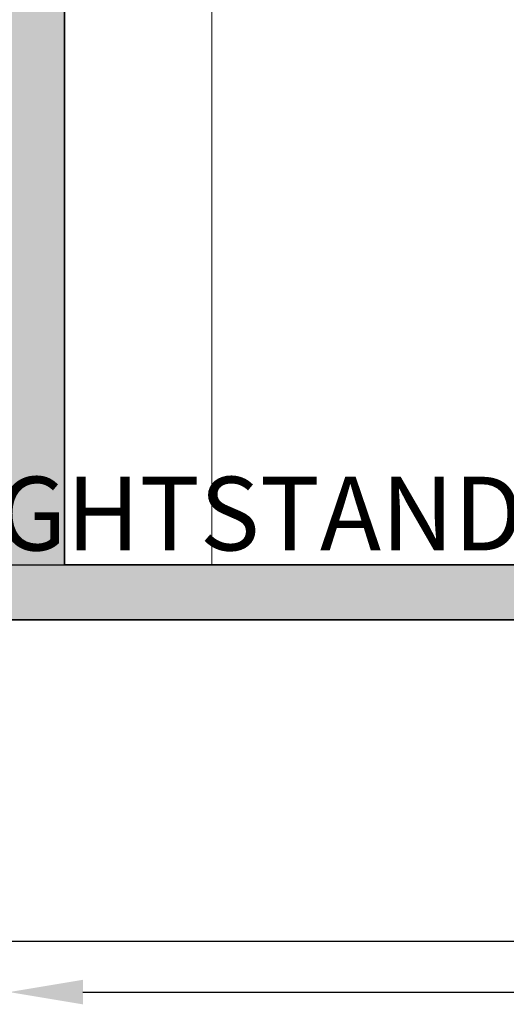
# Model space of a CAD drawing. Units: inches. Extents: x 2083 to 3317, y 1141 to 2115.
# Tile 111 of 256: x 2865 to 2944, y 1201 to 1361. Entities that reach past the tile are written whole.
import ezdxf

# ---------------------------------------------------------------- set-up
doc = ezdxf.new("R2010")
doc.units = ezdxf.units.IN
for name, color, linetype, lineweight in [('A-ANNO-DIMS', 2, 'Continuous', 18), ('A-FLOR-CASE', 8, 'Continuous', 18), ('A-WALL', 7, 'Continuous', 35)]:
    doc.layers.add(name, color=color, linetype=linetype, lineweight=lineweight)
doc.layers.add('A-WALL-PATT', color=251, linetype='Continuous', lineweight=13, true_color=0x636466)
doc.styles.get("Standard").update_dxf_attribs({"font": 'arial.ttf'})
doc.dimstyles.new('ISO-25', dxfattribs={"dimtxt": 12, "dimasz": 12, "dimexe": 1.25, "dimexo": 0.625, "dimtad": 1, "dimlunit": 3, "dimtxsty": 'Standard', "dimcen": 2.5, "dimadec": 0, "dimazin": 0, "dimtfac": 1, "dimtmove": 0, "dimatfit": 3, "dimfxl": 1, "dimarcsym": 0})

# ---------------------------------------------------------------- blocks, each defined once
blk = doc.blocks.new('*D10')
at = {"layer": 'A-ANNO-DIMS', "color": 0, "lineweight": -2, "transparency": 16777216}
for p, q in [((2862.96, 1262.64), (2862.96, 1201.38)), ((3126.96, 1262.64), (3126.96, 1201.38)), ((2874.96, 1202.63), (3114.96, 1202.63))]:
    blk.add_line(p, q, dxfattribs=at)
at = {"layer": 'A-ANNO-DIMS', "color": 0, "transparency": 16777216}
for points in [[(2874.96, 1204.63), (2874.96, 1200.63), (2862.96, 1202.63)], [(3114.96, 1204.63), (3114.96, 1200.63), (3126.96, 1202.63)]]:
    blk.add_solid(points, dxfattribs=at)
at = {"layer": 'Defpoints', "color": 0, "transparency": 16777216}
for p in [(2862.96, 1263.26), (3126.96, 1263.26), (3126.96, 1202.63)]:
    blk.add_point(p, dxfattribs=at)
at = {"layer": 'A-ANNO-DIMS', "color": 0, "transparency": 16777216, "insert": (2994.96, 1209.28), "char_height": 12, "attachment_point": 5}
blk.add_mtext("22'", dxfattribs=at)
blk = doc.blocks.new('CASEWORK-96X24')
for q in [(0, 0), (24, 96)]:
    blk.add_line((0, 96), q)
blk = doc.blocks.new('*D26')
at = {"layer": 'A-ANNO-DIMS', "color": 0, "lineweight": -2, "transparency": 16777216}
for p, q in [((3088.99, 1274.92), (3088.99, 1270.95)), ((3111.24, 1274.92), (3111.24, 1270.95)), ((3076.99, 1272.2), (2840.26, 1272.2)), ((3111.24, 1272.2), (3088.99, 1272.2)), ((3123.24, 1272.2), (3135.24, 1272.2))]:
    blk.add_line(p, q, dxfattribs=at)
at = {"layer": 'A-ANNO-DIMS', "color": 0, "transparency": 16777216}
for points in [[(3076.99, 1274.2), (3076.99, 1270.2), (3088.99, 1272.2)], [(3123.24, 1274.2), (3123.24, 1270.2), (3111.24, 1272.2)]]:
    blk.add_solid(points, dxfattribs=at)
at = {"layer": 'Defpoints', "color": 0, "transparency": 16777216}
for p in [(3088.99, 1275.54), (3111.24, 1275.54), (3088.99, 1272.2)]:
    blk.add_point(p, dxfattribs=at)
at = {"layer": 'A-ANNO-DIMS', "color": 0, "transparency": 16777216, "insert": (2952.62, 1279.03), "char_height": 12, "attachment_point": 5}
blk.add_mtext('NIGHTSTAND 1\'-10 1/2" TYP.', dxfattribs=at)
blk = doc.blocks.new('*D34')
at = {"layer": 'A-ANNO-DIMS', "color": 0, "lineweight": -2, "transparency": 16777216}
for p, q in [((2226.96, 1262.64), (2226.96, 1209.66)), ((3126.96, 1262.64), (3126.96, 1209.66)), ((2238.96, 1210.91), (3114.96, 1210.91))]:
    blk.add_line(p, q, dxfattribs=at)
at = {"layer": 'A-ANNO-DIMS', "color": 0, "transparency": 16777216}
for points in [[(2238.96, 1212.91), (2238.96, 1208.91), (2226.96, 1210.91)], [(3114.96, 1212.91), (3114.96, 1208.91), (3126.96, 1210.91)]]:
    blk.add_solid(points, dxfattribs=at)
at = {"layer": 'Defpoints', "color": 0, "transparency": 16777216}
for p in [(2226.96, 1263.26), (3126.96, 1263.26), (3126.96, 1210.91)]:
    blk.add_point(p, dxfattribs=at)
at = {"layer": 'A-ANNO-DIMS', "color": 0, "transparency": 16777216, "insert": (2676.96, 1217.66), "char_height": 12, "attachment_point": 5}
blk.add_mtext('75\'-0"', dxfattribs=at)
blk = doc.blocks.new('*D73')
at = {"layer": 'A-ANNO-DIMS', "color": 0, "lineweight": -2, "transparency": 16777216}
for p, q in [((2895.87, 1420.76), (2930.55, 1387.52)), ((2980.11, 1340.03), (2939.22, 1379.22))]:
    blk.add_line(p, q, dxfattribs=at)
at = {"layer": 'A-ANNO-DIMS', "color": 0, "transparency": 16777216}
blk.add_solid([(2940.6, 1380.66), (2937.83, 1377.77), (2930.55, 1387.52)], dxfattribs=at)
at = {"layer": 'Defpoints', "color": 0, "transparency": 16777216}
for p in [(2895.87, 1420.76), (2930.55, 1387.52)]:
    blk.add_point(p, dxfattribs=at)
at = {"layer": 'A-ANNO-DIMS', "color": 0, "transparency": 16777216, "insert": (2968.66, 1360.35), "char_height": 12, "attachment_point": 5, "rotation": 316.2187}
blk.add_mtext('R4\'-0"', dxfattribs=at)

msp = doc.modelspace()

# ---------------------------------------------------------------- hatches: boundary and pattern name
at = {"layer": 'A-WALL-PATT'}
h = msp.add_hatch(color=256, dxfattribs=at)
h.dxf.hatch_style = 1
h.paths.add_polyline_path([(3126.96, 2020.761), (2748.96, 2020.761), (2604.96, 2020.761), (2226.96, 2020.761), (2226.96, 1702.761), (2466.96, 1702.761), (2466.96, 1582.761), (2418.96, 1582.761), (2418.96, 1477.761), (2226.96, 1477.761), (2226.96, 1263.261), (2544.96, 1263.261), (2544.96, 1411.761), (2604.96, 1411.761), (2685.96, 1411.761), (2685.96, 1420.761), (2604.96, 1420.761), (2604.96, 1573.761), (2604.96, 1702.761), (2604.96, 2011.761), (2748.96, 2011.761), (2748.96, 1702.761), (2862.96, 1702.761), (2862.96, 1621.761), (2871.96, 1621.761), (2871.96, 1702.761), (2883.96, 1702.761), (2883.96, 1706.939, -0.0264593), (2883.96, 1711.761), (2757.96, 1711.761), (2757.96, 1807.761), (2787.96, 1807.761), (2787.96, 1812.261), (2757.96, 1812.261), (2757.96, 2011.761), (2877.96, 2011.761), (2877.96, 1812.261), (2847.96, 1812.261), (2847.96, 1807.761), (2889.836, 1807.761), (2889.836, 1812.261), (2882.46, 1812.261), (2882.46, 2011.761), (3117.96, 2011.761), (3117.96, 1812.261), (2937.836, 1812.261), (2937.836, 1807.761), (2995.71, 1807.761), (2995.71, 1796.118), (3000.21, 1796.118), (3000.21, 1807.761), (3117.96, 1807.761), (3117.96, 1711.761), (3000.21, 1711.761), (3000.21, 1760.118), (2998.573, 1760.118, -0.020711), (2995.71, 1760.118), (2995.71, 1711.761), (2931.96, 1711.761), (2931.96, 1702.761), (3126.96, 1702.761)])
h.paths.add_polyline_path([(2471.46, 2011.761), (2471.46, 1810.011), (2462.717, 1810.011), (2462.717, 1805.511), (2505.96, 1805.511), (2505.96, 1810.011), (2475.96, 1810.011), (2475.96, 2011.761), (2595.96, 2011.761), (2595.96, 1810.011), (2565.96, 1810.011), (2565.96, 1805.511), (2595.96, 1805.511), (2595.96, 1711.761), (2235.96, 1711.761), (2235.96, 1805.511), (2353.71, 1805.511), (2353.71, 1796.054), (2358.21, 1796.054), (2358.21, 1805.511), (2414.717, 1805.511), (2414.717, 1810.011), (2235.96, 1810.011), (2235.96, 2011.761)], flags=16)
h.paths.add_polyline_path([(2270.205, 1994.61), (2270.205, 1970.61), (2246.205, 1970.61), (2246.205, 1994.61)], flags=0)
edge = h.paths.add_edge_path(flags=0)
edge.add_ellipse((2332.027, 1899.798), major_axis=(-3.043, 3.043), ratio=0.1682525, start_angle=-161.33217, end_angle=-156.30711, ccw=False)
edge.add_ellipse((2333.082, 1898.744), major_axis=(-1.055, 1.055), ratio=0.4535321, start_angle=-123.37102, end_angle=-94.15911)
edge = h.paths.add_edge_path(flags=0)
edge.add_ellipse((2332.027, 1968.876), major_axis=(3.043, 3.043), ratio=0.1682525, start_angle=18.66783, end_angle=23.69289)
edge.add_spline(control_points=[(2332.926, 1970.691), (2332.227, 1970.336), (2330.894, 1969.659), (2328.413, 1970.932), (2327.204, 1967.749), (2324.71, 1969.956), (2322.533, 1967.012), (2320.013, 1971.296), (2317.68, 1968.158), (2316.041, 1967.102), (2315.427, 1966.81)], knot_values=[0, 0, 0, 0, 2.2670587, 4.3245589, 6.6855835, 8.8786411, 11.121502, 14.300359, 17.7552837, 19.732645, 19.732645, 19.732645, 19.732645], degree=3, periodic=0)
edge.add_ellipse((2332.027, 1968.876), major_axis=(3.043, 3.043), ratio=0.1682525, start_angle=18.66783, end_angle=23.69289, ccw=False)
edge.add_ellipse((2333.082, 1969.931), major_axis=(1.055, 1.055), ratio=0.4535321, start_angle=56.62898, end_angle=85.84089, ccw=False)
edge = h.paths.add_edge_path(flags=0)
edge.add_spline(control_points=[(2296.428, 1967.988), (2293.628, 1965.336), (2287.704, 1959.727), (2299.744, 1949.996), (2294.533, 1935.669), (2290.573, 1920.604), (2293.394, 1909.974), (2296.185, 1904.967)], knot_values=[0.0991853, 0.0991853, 0.0991853, 0.0991853, 0.3453009, 0.6198217, 0.9826526, 1.3860932, 1.8105546, 1.8105546, 1.8105546, 1.8105546], degree=3, periodic=0)
edge.add_spline(control_points=[(2296.185, 1904.967), (2297.384, 1902.619), (2298.001, 1901.949), (2298.553, 1901.468)], knot_values=[0.0062457, 0.0062457, 0.0062457, 0.0062457, 0.0554759, 0.0554759, 0.0554759, 0.0554759], degree=3, periodic=0)
edge.add_spline(control_points=[(2298.553, 1901.468), (2297.259, 1900.923), (2295.225, 1900.232), (2293.06, 1900.614), (2292.101, 1900.788), (2292.09, 1900.791)], knot_values=[0.3128349, 0.3128349, 0.3128349, 0.3128349, 0.4017797, 0.4749867, 0.4759027, 0.4759027, 0.4759027, 0.4759027], degree=3, periodic=0)
edge.add_arc((2292.794, 1904.664), 3.937, 215.4209, 259.69818, ccw=False)
edge.add_spline(control_points=[(2289.585, 1902.382), (2289.477, 1902.535), (2289.368, 1902.688), (2289.261, 1902.841)], knot_values=[0.1028719, 0.1028719, 0.1028719, 0.1028719, 0.1168958, 0.1168958, 0.1168958, 0.1168958], degree=3, periodic=0)
edge.add_spline(control_points=[(2289.261, 1902.841), (2288.687, 1902.55), (2287.64, 1902.02), (2285.881, 1901.874), (2283.853, 1901.504), (2281.72, 1899.711), (2278.467, 1899.493), (2276.157, 1901.883), (2272.259, 1899.804), (2267.778, 1901.843), (2262.244, 1900.184), (2257.415, 1901.782), (2254.318, 1900.726), (2253.178, 1900.337)], knot_values=[0, 0, 0, 0, 1.9079767, 3.4771759, 5.261074, 7.9728515, 11.6802485, 13.7179214, 16.9395917, 22.789562, 27.5025027, 33.5952153, 37.1456181, 37.1456181, 37.1456181, 37.1456181], degree=3, periodic=0)
edge.add_line((2253.178, 1900.337), (2250.244, 1902.841))
edge.add_line((2250.244, 1902.841), (2250.244, 1965.833))
edge.add_line((2250.244, 1965.833), (2253.178, 1968.337))
edge.add_spline(control_points=[(2253.178, 1968.337), (2254.318, 1967.948), (2257.415, 1966.892), (2262.244, 1968.49), (2267.778, 1966.831), (2271.527, 1968.537), (2273.876, 1967.828), (2274.207, 1967.728)], knot_values=[0, 0, 0, 0, 0.0901802, 0.2449351, 0.3646438, 0.5132331, 0.5378548, 0.5378548, 0.5378548, 0.5378548], degree=3, periodic=0)
edge.add_arc((2274.353, 1963.793), 3.937, 72.05113, 92.12795, ccw=False)
edge.add_arc((2281.297, 1985.23), 18.596, 252.05113, 288.56572)
edge.add_arc((2292.317, 1956.029), 12.646, 71.02679, 113.77822, ccw=False)
edge = h.paths.add_edge_path(flags=0)
edge.add_spline(control_points=[(2274.899, 1951.856), (2275.066, 1951.617), (2275.233, 1951.377), (2275.398, 1951.136)], knot_values=[1.4099157, 1.4099157, 1.4099157, 1.4099157, 1.4315903, 1.4315903, 1.4315903, 1.4315903], degree=3, periodic=0)
edge.add_spline(control_points=[(2275.398, 1951.136), (2275.792, 1950.562), (2276.179, 1949.984), (2276.546, 1949.397)], knot_values=[1.3582378, 1.3582378, 1.3582378, 1.3582378, 1.4099157, 1.4099157, 1.4099157, 1.4099157], degree=3, periodic=0)
edge.add_line((2276.546, 1949.397), (2277.437, 1947.862))
edge.add_spline(control_points=[(2277.437, 1947.862), (2276.304, 1945.673), (2274.64, 1942.427), (2274.632, 1938.094), (2272.799, 1930.852), (2274.356, 1943.897), (2275.948, 1947.923), (2276.546, 1949.397)], knot_values=[0.0056315, 0.0056315, 0.0056315, 0.0056315, 0.1860139, 0.2660015, 0.3570872, 0.5963902, 0.7397317, 0.7397317, 0.7397317, 0.7397317], degree=3, periodic=0)
edge.add_spline(control_points=[(2276.546, 1949.397), (2276.179, 1949.984), (2275.792, 1950.562), (2275.398, 1951.136)], knot_values=[1.3582378, 1.3582378, 1.3582378, 1.3582378, 1.4099157, 1.4099157, 1.4099157, 1.4099157], degree=3, periodic=0)
edge.add_spline(control_points=[(2275.398, 1951.136), (2274.943, 1950.08), (2274.208, 1948.025), (2273.935, 1944.851), (2272.469, 1937.627), (2273.466, 1945.696), (2274.701, 1951.059), (2274.899, 1951.856)], knot_values=[0.1043639, 0.1043639, 0.1043639, 0.1043639, 0.1896363, 0.2696239, 0.3607096, 0.6000126, 0.6446217, 0.6446217, 0.6446217, 0.6446217], degree=3, periodic=0)
h.paths.add_polyline_path([(2269.168, 1963.128, -0.3575267), (2268.171, 1960.976, -0.0925607), (2268.171, 1939.436, -0.3575267), (2269.168, 1937.285, -0.3575267), (2267.016, 1938.282, -0.1647847), (2254.686, 1938.282, -0.3575267), (2252.534, 1937.285, -0.3575267), (2253.531, 1939.436, -0.0925607), (2253.531, 1960.976, -0.3575267), (2252.534, 1963.128, -0.3575267), (2254.686, 1962.131, -0.1647847), (2267.016, 1962.131, -0.3575267)], flags=0)
h.paths.add_polyline_path([(2248.874, 1967.802), (2248.874, 1957.028), (2249.458, 1957.028), (2249.458, 1911.647), (2248.874, 1911.647), (2248.874, 1900.873), (2246.512, 1900.873, 0.1973271), (2244.15, 1902.457), (2244.15, 1966.218, 0.1973271), (2246.512, 1967.802)], flags=0)
h.paths.add_polyline_path([(2269.168, 1931.389, -0.3575267), (2268.171, 1929.238, -0.0925607), (2268.171, 1907.698, -0.3575267), (2269.168, 1905.547, -0.3575267), (2267.016, 1906.544, -0.1647847), (2254.686, 1906.544, -0.3575267), (2252.534, 1905.547, -0.3575267), (2253.531, 1907.698, -0.0925607), (2253.531, 1929.238, -0.3575267), (2252.534, 1931.389, -0.3575267), (2254.686, 1930.392, -0.1647847), (2267.016, 1930.392, -0.3575267)], flags=0)
edge = h.paths.add_edge_path(flags=0)
edge.add_spline(control_points=[(2276.197, 1906.724), (2276.168, 1909.029), (2276.114, 1913.372), (2270.598, 1924.925), (2273.905, 1919.013), (2275.922, 1916.262), (2275.475, 1912.402), (2277.258, 1910.381), (2276.696, 1908.225), (2276.646, 1906.813), (2276.618, 1906.008)], knot_values=[0, 0, 0, 0, 8.6102597, 16.2212739, 18.8430575, 23.8048978, 27.4408283, 29.3561016, 31.2034776, 33.6506866, 33.6506866, 33.6506866, 33.6506866], degree=3, periodic=0)
edge.add_spline(control_points=[(2276.618, 1906.008), (2276.623, 1905.624), (2276.498, 1904.629), (2275.442, 1903.855), (2274.937, 1903.08), (2274.859, 1902.841)], knot_values=[0.1564884, 0.1564884, 0.1564884, 0.1564884, 0.1843975, 0.2313765, 0.2505985, 0.2505985, 0.2505985, 0.2505985], degree=3, periodic=0)
edge.add_line((2274.859, 1902.841), (2276.506, 1902.841))
edge.add_spline(control_points=[(2276.506, 1902.841), (2276.788, 1903.085), (2277.665, 1904.125), (2278.25, 1904.341), (2277.654, 1908.527), (2278.156, 1906.228), (2278.1, 1905.286), (2278.847, 1904.069), (2277.857, 1903.415), (2277.874, 1902.991), (2277.904, 1902.841)], knot_values=[0.0595743, 0.0595743, 0.0595743, 0.0595743, 0.0807529, 0.1037415, 0.1697201, 0.1760361, 0.2071372, 0.2404744, 0.2623409, 0.2736605, 0.2736605, 0.2736605, 0.2736605], degree=3, periodic=0)
edge.add_line((2277.904, 1902.841), (2280.03, 1902.841))
edge.add_spline(control_points=[(2280.03, 1902.841), (2279.888, 1903.088), (2279.499, 1903.982), (2280.152, 1905.939), (2278.104, 1909.658), (2279.762, 1907.185), (2280.328, 1904.875), (2280.485, 1903.49), (2281.463, 1903.249), (2281.758, 1902.936), (2281.834, 1902.841)], knot_values=[0.013856, 0.013856, 0.013856, 0.013856, 0.0348738, 0.0888667, 0.1078792, 0.1267378, 0.158714, 0.1937575, 0.2174868, 0.2267221, 0.2267221, 0.2267221, 0.2267221], degree=3, periodic=0)
edge.add_spline(control_points=[(2281.834, 1902.841), (2281.788, 1902.827), (2281.647, 1902.783), (2281.396, 1902.859), (2281.088, 1902.985), (2280.721, 1903.061), (2280.333, 1903.026), (2280.125, 1902.899), (2280.03, 1902.841)], knot_values=[0, 0, 0, 0, 0.1441304, 0.435517, 0.7492759, 1.1530457, 1.5483707, 1.878348, 1.878348, 1.878348, 1.878348], degree=3, periodic=0)
edge.add_line((2280.03, 1902.841), (2277.904, 1902.841))
edge.add_spline(control_points=[(2277.904, 1902.841), (2277.893, 1902.796), (2277.865, 1902.68), (2277.607, 1902.687), (2277.274, 1902.801), (2276.838, 1902.62), (2276.584, 1902.789), (2276.506, 1902.841)], knot_values=[0, 0, 0, 0, 0.1271885, 0.3261988, 0.6280094, 1.2435704, 1.5153306, 1.5153306, 1.5153306, 1.5153306], degree=3, periodic=0)
edge.add_line((2276.506, 1902.841), (2274.859, 1902.841))
edge.add_spline(control_points=[(2274.859, 1902.841), (2274.814, 1902.899), (2274.725, 1903.013), (2274.493, 1903.119), (2274.244, 1902.961), (2273.937, 1903.185), (2273.614, 1902.983), (2273.408, 1902.883), (2273.322, 1902.841)], knot_values=[0, 0, 0, 0, 0.2184302, 0.4369566, 0.6879766, 0.9903786, 1.3983955, 1.6918498, 1.6918498, 1.6918498, 1.6918498], degree=3, periodic=0)
edge.add_spline(control_points=[(2273.322, 1902.841), (2273.617, 1903.446), (2274.274, 1904.538), (2276.027, 1904.574), (2276.207, 1906.584), (2276.197, 1906.724)], knot_values=[0.0122268, 0.0122268, 0.0122268, 0.0122268, 0.0594721, 0.1062177, 0.134458, 0.134458, 0.134458, 0.134458], degree=3, periodic=0)
h.paths.add_polyline_path([(2270.776, 1897.79), (2270.776, 1873.79), (2246.776, 1873.79), (2246.776, 1897.79)], flags=0)
h.paths.add_polyline_path([(2353.71, 1760.005), (2353.71, 1760.054), (2358.21, 1760.054, -0.033729)], flags=0)
h.paths.add_polyline_path([(2321.819, 1737.529), (2341.995, 1737.529, -0.4142136), (2343.203, 1736.321), (2343.203, 1721.021, -0.4142136), (2341.995, 1719.813), (2321.819, 1719.813, -0.4142136), (2320.611, 1721.021), (2320.611, 1736.321, -0.4142136)], flags=0)
h.paths.add_polyline_path([(2324.235, 1736.321), (2339.579, 1736.321, -0.4142136), (2341.995, 1733.905), (2341.995, 1725.45, -0.4142136), (2339.579, 1723.034), (2333.681, 1723.034), (2333.845, 1722.045, -0.8706461), (2335.425, 1721.826, -0.767327), (2333.923, 1721.423), (2331.291, 1721.423, -0.767327), (2329.788, 1721.826, -0.8706461), (2331.368, 1722.045), (2331.533, 1723.034), (2324.235, 1723.034, -0.4142136), (2321.819, 1725.45), (2321.819, 1733.905, -0.4142136)], flags=0)
h.paths.add_polyline_path([(2570.484, 1928.615), (2589.684, 1928.615), (2590.169, 1928.615), (2590.169, 1904.993), (2570.484, 1904.993)], flags=0)
h.paths.add_polyline_path([(2574.447, 1927.264, -1), (2572.829, 1927.264, -1)], flags=0)
h.paths.add_polyline_path([(2573.09, 1926.941), (2573.925, 1927.776), (2574.148, 1927.553), (2573.313, 1926.718)], flags=0)
h.paths.add_polyline_path([(2578.779, 1919.73, -1), (2571.592, 1919.73, -1)], flags=0)
h.paths.add_polyline_path([(2578.385, 1919.73, -1), (2571.985, 1919.73, -1)], flags=0)
h.paths.add_polyline_path([(2331.596, 1729.476, -1), (2333.618, 1729.476, -1)], flags=0)
h.paths.add_polyline_path([(2578.034, 1927.264, -1), (2576.416, 1927.264, -1)], flags=0)
h.paths.add_polyline_path([(2576.689, 1927.531), (2576.912, 1927.754), (2577.747, 1926.919), (2577.524, 1926.696)], flags=0)
h.paths.add_polyline_path([(2578.139, 1909.86, -1), (2572.232, 1909.86, -1)], flags=0)
h.paths.add_polyline_path([(2577.745, 1909.86, -1), (2572.625, 1909.86, -1)], flags=0)
h.paths.add_polyline_path([(2583.798, 1927.264, -1), (2582.179, 1927.264, -1)], flags=0)
h.paths.add_polyline_path([(2582.719, 1927.754), (2583.554, 1926.919), (2583.331, 1926.696), (2582.496, 1927.531)], flags=0)
h.paths.add_polyline_path([(2582.496, 1927.531), (2582.719, 1927.754), (2583.554, 1926.919), (2583.331, 1926.696)], flags=0)
h.paths.add_polyline_path([(2587.739, 1920.53, -1), (2581.832, 1920.53, -1)], flags=0)
h.paths.add_polyline_path([(2587.345, 1920.53, -1), (2582.225, 1920.53, -1)], flags=0)
h.paths.add_polyline_path([(2587.385, 1927.264, -1), (2585.766, 1927.264, -1)], flags=0)
h.paths.add_polyline_path([(2586.082, 1926.98), (2586.917, 1927.815), (2587.14, 1927.593), (2586.305, 1926.758)], flags=0)
h.paths.add_polyline_path([(2588.379, 1910.66, -1), (2581.192, 1910.66, -1)], flags=0)
h.paths.add_polyline_path([(2587.985, 1910.66, -1), (2581.585, 1910.66, -1)], flags=0)
h.paths.add_polyline_path([(2417.168, 1729.478), (2437.344, 1729.478, -0.4142136), (2438.552, 1728.27), (2438.552, 1712.969, -0.4142136), (2437.344, 1711.761), (2417.168, 1711.761, -0.4142136), (2415.96, 1712.969), (2415.96, 1728.27, -0.4142136)], flags=0)
h.paths.add_polyline_path([(2419.584, 1728.27), (2434.928, 1728.27, -0.4142136), (2437.344, 1725.854), (2437.344, 1717.398, -0.4142136), (2434.928, 1714.983), (2429.029, 1714.983), (2429.194, 1713.994, -0.8706461), (2430.774, 1713.775, -0.767327), (2429.271, 1713.372), (2426.64, 1713.372, -0.767327), (2425.137, 1713.775, -0.8706461), (2426.717, 1713.994), (2426.882, 1714.983), (2419.584, 1714.983, -0.4142136), (2417.168, 1717.398), (2417.168, 1725.854, -0.4142136)], flags=0)
h.paths.add_polyline_path([(2419.584, 1728.27), (2434.928, 1728.27, -0.4142136), (2437.344, 1725.854), (2437.344, 1717.398, -0.4142136), (2434.928, 1714.983), (2429.029, 1714.983), (2428.358, 1719.009), (2427.553, 1719.009), (2426.882, 1714.983), (2419.584, 1714.983, -0.4142136), (2417.168, 1717.398), (2417.168, 1725.854, -0.4142136)], flags=0)
h.paths.add_polyline_path([(2426.944, 1721.425, -1), (2428.967, 1721.425, -1)], flags=0)
h.paths.add_polyline_path([(2475.96, 1702.761), (2595.96, 1702.761), (2595.96, 1582.761), (2475.96, 1582.761)], flags=16)
h.paths.add_polyline_path([(2427.96, 1573.761), (2595.96, 1573.761), (2595.96, 1468.761), (2595.96, 1420.761), (2384.46, 1420.761), (2384.46, 1468.761), (2427.96, 1468.761)], flags=16)
h.paths.add_polyline_path([(2379.96, 1468.761), (2379.96, 1420.761), (2235.96, 1420.761), (2235.96, 1468.761)], flags=16)
h.paths.add_polyline_path([(2317.816, 1466.696), (2337.992, 1466.696, -0.4142136), (2339.2, 1465.488), (2339.2, 1450.187, -0.4142136), (2337.992, 1448.979), (2317.816, 1448.979, -0.4142136), (2316.608, 1450.187), (2316.608, 1465.488, -0.4142136)], flags=0)
h.paths.add_polyline_path([(2320.232, 1465.488), (2335.576, 1465.488, -0.4142136), (2337.992, 1463.072), (2337.992, 1454.616, -0.4142136), (2335.576, 1452.2), (2329.677, 1452.2), (2329.842, 1451.212, -0.8706461), (2331.422, 1450.992, -0.767327), (2329.92, 1450.59), (2327.288, 1450.59, -0.767327), (2325.785, 1450.992, -0.8706461), (2327.365, 1451.212), (2327.53, 1452.2), (2320.232, 1452.2, -0.4142136), (2317.816, 1454.616), (2317.816, 1463.072, -0.4142136)], flags=0)
h.paths.add_polyline_path([(2320.232, 1465.488), (2335.576, 1465.488, -0.4142136), (2337.992, 1463.072), (2337.992, 1454.616, -0.4142136), (2335.576, 1452.2), (2329.677, 1452.2), (2329.006, 1456.227), (2328.201, 1456.227), (2327.53, 1452.2), (2320.232, 1452.2, -0.4142136), (2317.816, 1454.616), (2317.816, 1463.072, -0.4142136)], flags=0)
h.paths.add_polyline_path([(2327.593, 1458.643, -1), (2329.615, 1458.643, -1)], flags=0)
h.paths.add_polyline_path([(2244.412, 1433.34), (2241.921, 1433.34, -0.4142136), (2240.018, 1435.244), (2240.018, 1440.953, -0.4142105), (2241.921, 1442.856), (2244.412, 1442.856, -1.9764724)], flags=0)
h.paths.add_polyline_path([(2245.357, 1434.398, -0.4142136), (2245.357, 1441.799, -2.1440985)], flags=0)
h.paths.add_polyline_path([(2535.96, 1416.261), (2535.96, 1272.261), (2235.96, 1272.261), (2235.96, 1416.261)], flags=16)
h.paths.add_polyline_path([(2260.12, 1384.293), (2260.12, 1362.039), (2237.865, 1362.039), (2237.865, 1384.293)], flags=0)
edge = h.paths.add_edge_path(flags=0)
edge.add_line((2318.252, 1362.093), (2318.146, 1362.001))
edge.add_ellipse((2317.445, 1360.431), major_axis=(2.822, 2.822), ratio=0.1682525, start_angle=18.66783, end_angle=20.94813, ccw=False)
edge.add_ellipse((2318.423, 1361.409), major_axis=(0.978, 0.978), ratio=0.4535321, start_angle=56.62898, end_angle=70.2262, ccw=False)
edge = h.paths.add_edge_path(flags=0)
edge.add_line((2319.107, 1295.571), (2319.015, 1295.677))
edge.add_ellipse((2317.445, 1296.378), major_axis=(-2.822, 2.822), ratio=0.1682525, start_angle=-161.33217, end_angle=-159.05187, ccw=False)
edge.add_ellipse((2318.423, 1295.4), major_axis=(-0.978, 0.978), ratio=0.4535321, start_angle=-123.37102, end_angle=-109.7738)
edge = h.paths.add_edge_path(flags=0)
edge.add_spline(control_points=[(2284.21, 1301.17), (2284.581, 1300.445), (2284.891, 1299.892), (2285.16, 1299.461)], knot_values=[0.0390658, 0.0390658, 0.0390658, 0.0390658, 0.0554759, 0.0554759, 0.0554759, 0.0554759], degree=3, periodic=0)
edge.add_line((2285.16, 1299.461), (2284.21, 1301.17))
edge = h.paths.add_edge_path(flags=0)
edge.add_line((2280.412, 1297.298), (2283.37, 1297.036))
edge.add_line((2283.37, 1297.036), (2286.406, 1297.926))
edge.add_spline(control_points=[(2286.406, 1297.926), (2285.305, 1297.463), (2284.345, 1297.129), (2283.37, 1297.036)], knot_values=[0.3943688, 0.3943688, 0.3943688, 0.3943688, 0.4759027, 0.4759027, 0.4759027, 0.4759027], degree=3, periodic=0)
edge.add_spline(control_points=[(2283.37, 1297.036), (2283.281, 1297.028), (2282.316, 1296.957), (2281.313, 1297.134), (2280.423, 1297.296), (2280.412, 1297.298)], knot_values=[0.3128349, 0.3128349, 0.3128349, 0.3128349, 0.3202458, 0.3934528, 0.3943688, 0.3943688, 0.3943688, 0.3943688], degree=3, periodic=0)
edge = h.paths.add_edge_path(flags=0)
edge.add_line((2284.436, 1359.607), (2280.446, 1355.328))
edge.add_line((2280.446, 1355.328), (2279.58, 1351.018))
edge.add_line((2279.58, 1351.018), (2282.413, 1346.58))
edge.add_spline(control_points=[(2282.413, 1346.58), (2283.153, 1345.589), (2284.253, 1344.029), (2284.801, 1342.387), (2284.935, 1341.806)], knot_values=[1.2400982, 1.2400982, 1.2400982, 1.2400982, 1.3328922, 1.3827123, 1.3827123, 1.3827123, 1.3827123], degree=3, periodic=0)
edge.add_spline(control_points=[(2284.935, 1341.806), (2285.319, 1340.141), (2285.233, 1338.409), (2284.91, 1336.654)], knot_values=[1.0974841, 1.0974841, 1.0974841, 1.0974841, 1.2400982, 1.2400982, 1.2400982, 1.2400982], degree=3, periodic=0)
edge.add_spline(control_points=[(2284.91, 1336.654), (2284.587, 1334.899), (2284.027, 1333.12), (2283.463, 1331.361)], knot_values=[0.9548699, 0.9548699, 0.9548699, 0.9548699, 1.0974841, 1.0974841, 1.0974841, 1.0974841], degree=3, periodic=0)
edge.add_line((2283.463, 1331.361), (2281.89, 1326.153))
edge.add_line((2281.89, 1326.153), (2280.756, 1321.056))
edge.add_line((2280.756, 1321.056), (2280.299, 1316.002))
edge.add_line((2280.299, 1316.002), (2280.716, 1310.95))
edge.add_line((2280.716, 1310.95), (2282.028, 1305.972))
edge.add_line((2282.028, 1305.972), (2284.21, 1301.17))
edge.add_spline(control_points=[(2284.21, 1301.17), (2283.341, 1302.73), (2282.612, 1304.336), (2282.028, 1305.972)], knot_values=[0.0991853, 0.0991853, 0.0991853, 0.0991853, 0.2417994, 0.2417994, 0.2417994, 0.2417994], degree=3, periodic=0)
edge.add_spline(control_points=[(2282.028, 1305.972), (2281.444, 1307.608), (2281.005, 1309.273), (2280.716, 1310.95)], knot_values=[0.2417994, 0.2417994, 0.2417994, 0.2417994, 0.3844135, 0.3844135, 0.3844135, 0.3844135], degree=3, periodic=0)
edge.add_spline(control_points=[(2280.716, 1310.95), (2280.433, 1312.588), (2280.289, 1314.277), (2280.299, 1315.962), (2280.299, 1316.002)], knot_values=[0.3844135, 0.3844135, 0.3844135, 0.3844135, 0.5236467, 0.5270276, 0.5270276, 0.5270276, 0.5270276], degree=3, periodic=0)
edge.add_spline(control_points=[(2280.299, 1316.002), (2280.312, 1317.687), (2280.478, 1319.368), (2280.756, 1321.056)], knot_values=[0.5270276, 0.5270276, 0.5270276, 0.5270276, 0.6696417, 0.6696417, 0.6696417, 0.6696417], degree=3, periodic=0)
edge.add_spline(control_points=[(2280.756, 1321.056), (2281.035, 1322.744), (2281.426, 1324.44), (2281.89, 1326.153)], knot_values=[0.6696417, 0.6696417, 0.6696417, 0.6696417, 0.8122558, 0.8122558, 0.8122558, 0.8122558], degree=3, periodic=0)
edge.add_spline(control_points=[(2281.89, 1326.153), (2282.264, 1327.533), (2282.788, 1329.262), (2283.353, 1331.018), (2283.463, 1331.361)], knot_values=[0.8122558, 0.8122558, 0.8122558, 0.8122558, 0.9270873, 0.9548699, 0.9548699, 0.9548699, 0.9548699], degree=3, periodic=0)
edge.add_line((2283.463, 1331.361), (2284.91, 1336.654))
edge.add_line((2284.91, 1336.654), (2284.935, 1341.806))
edge.add_line((2284.935, 1341.806), (2282.413, 1346.58))
edge.add_spline(control_points=[(2282.413, 1346.58), (2281.275, 1348.104), (2280.078, 1349.57), (2279.58, 1351.018)], knot_values=[1.3827123, 1.3827123, 1.3827123, 1.3827123, 1.5253264, 1.5253264, 1.5253264, 1.5253264], degree=3, periodic=0)
edge.add_spline(control_points=[(2279.58, 1351.018), (2279.443, 1351.415), (2279.136, 1352.857), (2279.735, 1354.29), (2280.446, 1355.328)], knot_values=[1.5253264, 1.5253264, 1.5253264, 1.5253264, 1.564439, 1.6679405, 1.6679405, 1.6679405, 1.6679405], degree=3, periodic=0)
edge.add_spline(control_points=[(2280.446, 1355.328), (2281.426, 1356.758), (2282.931, 1358.183), (2284.436, 1359.607)], knot_values=[1.6679405, 1.6679405, 1.6679405, 1.6679405, 1.8105546, 1.8105546, 1.8105546, 1.8105546], degree=3, periodic=0)
edge.add_arc((2280.623, 1348.518), 11.726, 71.02679, 113.77822)
edge.add_arc((2270.405, 1375.595), 17.244, 252.05113, 288.56572, ccw=False)
edge.add_arc((2263.966, 1355.718), 3.651, 72.05113, 92.12795)
edge.add_arc((2263.966, 1355.718), 3.651, 92.12795, 177.98513)
edge.add_spline(control_points=[(2260.318, 1355.846), (2260.26, 1354.221), (2260.551, 1350.187), (2262.999, 1346.766), (2264.473, 1344.649)], knot_values=[1.4315903, 1.4315903, 1.4315903, 1.4315903, 1.5641438, 1.7706953, 1.7706953, 1.7706953, 1.7706953], degree=3, periodic=0)
edge.add_line((2264.473, 1344.649), (2264.936, 1343.983))
edge.add_spline(control_points=[(2263.801, 1340.248), (2263.843, 1340.514), (2264.067, 1341.756), (2264.513, 1343.002), (2264.935, 1343.981)], knot_values=[0.5365702, 0.5365702, 0.5365702, 0.5365702, 0.5593494, 0.6446217, 0.6446217, 0.6446217, 0.6446217], degree=3, periodic=0)
edge.add_spline(control_points=[(2264.935, 1343.981), (2265.118, 1343.715), (2265.299, 1343.448), (2265.477, 1343.179)], knot_values=[1.3840767, 1.3840767, 1.3840767, 1.3840767, 1.4099157, 1.4099157, 1.4099157, 1.4099157], degree=3, periodic=0)
edge.add_spline(control_points=[(2265.477, 1343.179), (2265.655, 1342.911), (2265.829, 1342.641), (2265.999, 1342.369)], knot_values=[1.3582378, 1.3582378, 1.3582378, 1.3582378, 1.3840767, 1.3840767, 1.3840767, 1.3840767], degree=3, periodic=0)
edge.add_line((2265.999, 1342.369), (2266.826, 1340.946))
edge.add_spline(control_points=[(2266.826, 1340.946), (2268.894, 1337.09), (2271.398, 1325.843), (2270.516, 1310.569), (2275.919, 1301.861), (2277.79, 1299.199)], knot_values=[0.1168958, 0.1168958, 0.1168958, 0.1168958, 0.4729873, 1.0509689, 1.3137934, 1.3137934, 1.3137934, 1.3137934], degree=3, periodic=0)
edge.add_spline(control_points=[(2277.79, 1299.199), (2277.839, 1299.128), (2277.889, 1299.057), (2277.94, 1298.987)], knot_values=[0.1098839, 0.1098839, 0.1098839, 0.1098839, 0.1168958, 0.1168958, 0.1168958, 0.1168958], degree=3, periodic=0)
edge.add_line((2277.94, 1298.987), (2277.789, 1299.199))
edge.add_spline(control_points=[(2277.789, 1299.199), (2277.257, 1298.929), (2276.286, 1298.438), (2275.039, 1298.334), (2274.383, 1298.239), (2274.215, 1298.209)], knot_values=[33.1218702, 33.1218702, 33.1218702, 33.1218702, 35.0290557, 36.5982549, 37.1448269, 37.1448269, 37.1448269, 37.1448269], degree=3, periodic=0)
edge.add_line((2274.215, 1298.209), (2273.073, 1297.893))
edge.add_spline(control_points=[(2273.073, 1297.893), (2272.323, 1297.58), (2271.039, 1296.511), (2269.248, 1296.226), (2268.423, 1296.375)], knot_values=[26.5325843, 26.5325843, 26.5325843, 26.5325843, 29.198919, 31.8391012, 31.8391012, 31.8391012, 31.8391012], degree=3, periodic=0)
edge.add_line((2268.423, 1296.375), (2263.879, 1297.458))
edge.add_spline(control_points=[(2263.879, 1297.458), (2263.556, 1297.359), (2261.86, 1296.839), (2260.239, 1297.282), (2258.933, 1297.516)], knot_values=[15.9195506, 15.9195506, 15.9195506, 15.9195506, 16.9395917, 21.2260675, 21.2260675, 21.2260675, 21.2260675], degree=3, periodic=0)
edge.add_line((2258.933, 1297.516), (2254.055, 1297.329))
edge.add_spline(control_points=[(2254.055, 1297.329), (2253.756, 1297.296), (2252.114, 1297.165), (2250.462, 1297.544), (2249.13, 1297.668)], knot_values=[5.3065169, 5.3065169, 5.3065169, 5.3065169, 6.2764352, 10.6130337, 10.6130337, 10.6130337, 10.6130337], degree=3, periodic=0)
edge.add_line((2249.13, 1297.668), (2244.332, 1296.878))
edge.add_line((2244.332, 1296.878), (2241.611, 1299.199))
edge.add_line((2241.611, 1299.199), (2241.611, 1357.609))
edge.add_line((2241.611, 1357.609), (2244.332, 1359.931))
edge.add_line((2244.332, 1359.931), (2252.729, 1359.543))
edge.add_spline(control_points=[(2252.729, 1359.543), (2252.871, 1359.546), (2253.306, 1359.548), (2253.74, 1359.514), (2254.032, 1359.482)], knot_values=[0.233291, 0.233291, 0.233291, 0.233291, 0.2449351, 0.2689274, 0.2689274, 0.2689274, 0.2689274], degree=3, periodic=0)
edge.add_line((2254.032, 1359.482), (2259.587, 1359.416))
edge.add_spline(control_points=[(2259.587, 1359.416), (2260.677, 1359.629), (2262.073, 1359.897), (2263.524, 1359.459), (2263.83, 1359.366)], knot_values=[0.4225164, 0.4225164, 0.4225164, 0.4225164, 0.5132331, 0.5378548, 0.5378548, 0.5378548, 0.5378548], degree=3, periodic=0)
edge.add_arc((2263.966, 1355.718), 3.651, 72.05113, 92.12795, ccw=False)
edge.add_arc((2270.405, 1375.595), 17.244, 252.05113, 288.56572)
edge.add_arc((2280.623, 1348.518), 11.726, 71.02679, 113.77822, ccw=False)
h.paths.add_polyline_path([(2240.341, 1359.435), (2240.341, 1349.444), (2240.882, 1349.444), (2240.882, 1307.365), (2240.341, 1307.365), (2240.341, 1297.374), (2238.15, 1297.374, 0.1973271), (2235.96, 1298.843), (2235.96, 1357.966, 0.1973271), (2238.15, 1359.435)], flags=0)
h.paths.add_polyline_path([(2259.158, 1355.101, -0.3575267), (2258.233, 1353.106, -0.0925607), (2258.233, 1333.133, -0.3575267), (2259.158, 1331.138, -0.3575267), (2257.163, 1332.062, -0.1647847), (2245.729, 1332.062, -0.3575267), (2243.735, 1331.138, -0.3575267), (2244.659, 1333.133, -0.0925607), (2244.659, 1353.106, -0.3575267), (2243.735, 1355.101, -0.3575267), (2245.729, 1354.176, -0.1647847), (2257.163, 1354.176, -0.3575267)], flags=0)
edge = h.paths.add_edge_path(flags=0)
edge.add_line((2265.999, 1342.369), (2266.826, 1340.946))
edge.add_line((2266.826, 1340.946), (2265.308, 1337.814))
edge.add_line((2265.308, 1337.814), (2264.358, 1334.653))
edge.add_line((2264.358, 1334.653), (2264.262, 1333.8))
edge.add_spline(control_points=[(2264.262, 1333.8), (2264.208, 1333.187), (2264.162, 1332.366), (2264.007, 1331.414), (2263.969, 1331.202)], knot_values=[0.4644442, 0.4644442, 0.4644442, 0.4644442, 0.5166905, 0.5316081, 0.5316081, 0.5316081, 0.5316081], degree=3, periodic=0)
edge.add_spline(control_points=[(2263.969, 1331.202), (2263.775, 1330.119), (2263.424, 1328.791), (2263.257, 1328.531), (2263.234, 1328.515)], knot_values=[0.3726816, 0.3726816, 0.3726816, 0.3726816, 0.4488497, 0.4644442, 0.4644442, 0.4644442, 0.4644442], degree=3, periodic=0)
edge.add_spline(control_points=[(2263.234, 1328.515), (2263.096, 1328.42), (2263.131, 1329.301), (2263.275, 1330.616)], knot_values=[0.2809191, 0.2809191, 0.2809191, 0.2809191, 0.3726816, 0.3726816, 0.3726816, 0.3726816], degree=3, periodic=0)
edge.add_spline(control_points=[(2263.275, 1330.616), (2263.419, 1331.93), (2263.672, 1333.677), (2263.97, 1335.315)], knot_values=[0.1891566, 0.1891566, 0.1891566, 0.1891566, 0.2809191, 0.2809191, 0.2809191, 0.2809191], degree=3, periodic=0)
edge.add_spline(control_points=[(2263.97, 1335.315), (2264.1, 1336.032), (2264.419, 1337.622), (2264.755, 1338.864), (2264.947, 1339.491)], knot_values=[0.097394, 0.097394, 0.097394, 0.097394, 0.1375775, 0.1891566, 0.1891566, 0.1891566, 0.1891566], degree=3, periodic=0)
edge.add_spline(control_points=[(2264.947, 1339.491), (2265.29, 1340.606), (2265.644, 1341.494), (2265.999, 1342.369)], knot_values=[0.0056315, 0.0056315, 0.0056315, 0.0056315, 0.097394, 0.097394, 0.097394, 0.097394], degree=3, periodic=0)
h.paths.add_polyline_path([(2259.158, 1325.671, -0.3575267), (2258.233, 1323.676, -0.0925607), (2258.233, 1303.703, -0.3575267), (2259.158, 1301.708, -0.3575267), (2257.163, 1302.633, -0.1647847), (2245.729, 1302.633, -0.3575267), (2243.735, 1301.708, -0.3575267), (2244.659, 1303.703, -0.0925607), (2244.659, 1323.676, -0.3575267), (2243.735, 1325.671, -0.3575267), (2245.729, 1324.747, -0.1647847), (2257.163, 1324.747, -0.3575267)], flags=0)
edge = h.paths.add_edge_path(flags=0)
edge.add_spline(control_points=[(2261.709, 1317.311), (2261.679, 1317.418), (2261.762, 1317.389), (2262.491, 1316.09), (2262.962, 1315.301)], knot_values=[14.9558607, 14.9558607, 14.9558607, 14.9558607, 16.2212739, 18.6948259, 18.6948259, 18.6948259, 18.6948259], degree=3, periodic=0)
edge.add_spline(control_points=[(2262.962, 1315.301), (2262.99, 1315.254), (2263.702, 1314.067), (2264.349, 1313.127), (2264.73, 1312.164)], knot_values=[18.6948259, 18.6948259, 18.6948259, 18.6948259, 18.8430575, 22.433791, 22.433791, 22.433791, 22.433791], degree=3, periodic=0)
edge.add_spline(control_points=[(2264.73, 1312.164), (2264.876, 1311.796), (2265.177, 1310.77), (2265.143, 1309.559), (2265.248, 1308.824)], knot_values=[22.433791, 22.433791, 22.433791, 22.433791, 23.8048978, 26.1727562, 26.1727562, 26.1727562, 26.1727562], degree=3, periodic=0)
edge.add_line((2265.248, 1308.824), (2265.851, 1307.172))
edge.add_spline(control_points=[(2265.851, 1307.172), (2266.065, 1306.822), (2266.384, 1306.332), (2266.424, 1305.781), (2266.42, 1305.611)], knot_values=[28.0625624, 28.0625624, 28.0625624, 28.0625624, 29.3561016, 29.9117214, 29.9117214, 29.9117214, 29.9117214], degree=3, periodic=0)
edge.add_spline(control_points=[(2266.42, 1305.611), (2266.416, 1305.433), (2266.394, 1305.25), (2266.365, 1305.066)], knot_values=[29.9117214, 29.9117214, 29.9117214, 29.9117214, 30.4978371, 30.4978371, 30.4978371, 30.4978371], degree=3, periodic=0)
edge.add_line((2266.365, 1305.066), (2266.066, 1302.136))
edge.add_spline(control_points=[(2266.066, 1302.136), (2266.071, 1301.78), (2265.998, 1301.2), (2265.663, 1300.759), (2265.509, 1300.586)], knot_values=[0.1564884, 0.1564884, 0.1564884, 0.1564884, 0.1843975, 0.2035434, 0.2035434, 0.2035434, 0.2035434], degree=3, periodic=0)
edge.add_line((2265.509, 1300.586), (2264.435, 1299.199))
edge.add_line((2264.435, 1299.199), (2265.962, 1299.199))
edge.add_line((2265.962, 1299.199), (2267.336, 1301.175))
edge.add_line((2267.336, 1301.175), (2267.312, 1301.986))
edge.add_spline(control_points=[(2267.312, 1301.986), (2267.261, 1302.862), (2267.16, 1303.737), (2267.271, 1303.326)], knot_values=[0.1262286, 0.1262286, 0.1262286, 0.1262286, 0.1666174, 0.1666174, 0.1666174, 0.1666174], degree=3, periodic=0)
edge.add_spline(control_points=[(2267.271, 1303.326), (2267.28, 1303.294), (2267.31, 1303.175), (2267.373, 1302.884), (2267.406, 1302.683), (2267.418, 1302.601)], knot_values=[0.1666174, 0.1666174, 0.1666174, 0.1666174, 0.1697201, 0.1760361, 0.1807647, 0.1807647, 0.1807647, 0.1807647], degree=3, periodic=0)
edge.add_spline(control_points=[(2267.744, 1300.988), (2267.688, 1301.151), (2267.481, 1301.657), (2267.484, 1302.145), (2267.418, 1302.601)], knot_values=[0.1807647, 0.1807647, 0.1807647, 0.1807647, 0.1937665, 0.2201389, 0.2201389, 0.2201389, 0.2201389], degree=3, periodic=0)
edge.add_line((2267.418, 1302.601), (2267.744, 1300.988))
edge.add_spline(control_points=[(2267.744, 1300.988), (2267.832, 1300.732), (2267.932, 1300.31), (2267.555, 1299.975), (2267.429, 1299.829)], knot_values=[0.2201389, 0.2201389, 0.2201389, 0.2201389, 0.2404744, 0.2548903, 0.2548903, 0.2548903, 0.2548903], degree=3, periodic=0)
edge.add_line((2267.429, 1299.829), (2267.258, 1299.199))
edge.add_line((2267.258, 1299.199), (2269.23, 1299.199))
edge.add_spline(control_points=[(2269.23, 1299.199), (2269.099, 1299.429), (2268.843, 1300.016), (2269.012, 1300.916), (2268.947, 1301.661)], knot_values=[0.013856, 0.013856, 0.013856, 0.013856, 0.0348738, 0.0670726, 0.0670726, 0.0670726, 0.0670726], degree=3, periodic=0)
edge.add_line((2268.947, 1301.661), (2268.432, 1303.603))
edge.add_spline(control_points=[(2268.432, 1303.603), (2268.176, 1304.192), (2267.596, 1305.251), (2268.041, 1304.623), (2268.251, 1304.282)], knot_values=[0.0901547, 0.0901547, 0.0901547, 0.0901547, 0.1078792, 0.1202891, 0.1202891, 0.1202891, 0.1202891], degree=3, periodic=0)
edge.add_spline(control_points=[(2268.251, 1304.282), (2268.361, 1304.105), (2269.058, 1302.918), (2269.383, 1301.59), (2269.521, 1300.776), (2269.575, 1300.556)], knot_values=[0.1202891, 0.1202891, 0.1202891, 0.1202891, 0.1267378, 0.158714, 0.1735056, 0.1735056, 0.1735056, 0.1735056], degree=3, periodic=0)
edge.add_line((2269.575, 1300.556), (2270.686, 1299.421))
edge.add_spline(control_points=[(2270.686, 1299.421), (2270.767, 1299.357), (2270.838, 1299.281), (2270.903, 1299.199)], knot_values=[0.2181597, 0.2181597, 0.2181597, 0.2181597, 0.2267221, 0.2267221, 0.2267221, 0.2267221], degree=3, periodic=0)
edge.add_line((2270.937, 1299.193), (2270.903, 1299.199))
edge.add_spline(control_points=[(2270.903, 1299.199), (2270.86, 1299.186), (2270.73, 1299.146), (2270.496, 1299.216), (2270.272, 1299.308), (2270.121, 1299.348), (2270.063, 1299.36)], knot_values=[0.939174, 0.939174, 0.939174, 0.939174, 1.0833044, 1.3746911, 1.6884499, 1.878348, 1.878348, 1.878348, 1.878348], degree=3, periodic=0)
edge.add_line((2270.063, 1299.36), (2269.23, 1299.199))
edge.add_line((2269.23, 1299.199), (2267.258, 1299.199))
edge.add_spline(control_points=[(2267.258, 1299.199), (2267.248, 1299.157), (2267.223, 1299.05), (2266.984, 1299.057), (2266.809, 1299.116), (2266.677, 1299.109), (2266.637, 1299.105)], knot_values=[0.7576653, 0.7576653, 0.7576653, 0.7576653, 0.8848538, 1.0838641, 1.3856747, 1.5153306, 1.5153306, 1.5153306, 1.5153306], degree=3, periodic=0)
edge.add_spline(control_points=[(2266.637, 1299.105), (2266.485, 1299.089), (2266.236, 1299.017), (2266.035, 1299.151), (2265.962, 1299.199)], knot_values=[0, 0, 0, 0, 0.4859051, 0.7576653, 0.7576653, 0.7576653, 0.7576653], degree=3, periodic=0)
edge.add_line((2265.962, 1299.199), (2264.435, 1299.199))
edge.add_line((2264.435, 1299.199), (2263.858, 1299.367))
edge.add_spline(control_points=[(2263.858, 1299.367), (2263.819, 1299.371), (2263.78, 1299.386), (2263.74, 1299.402)], knot_values=[0.8459249, 0.8459249, 0.8459249, 0.8459249, 0.9786272, 0.9786272, 0.9786272, 0.9786272], degree=3, periodic=0)
edge.add_line((2263.722, 1299.396), (2263.01, 1299.199))
edge.add_spline(control_points=[(2263.01, 1299.199), (2263.246, 1299.683), (2263.506, 1300.128), (2263.873, 1300.408)], knot_values=[0.0122268, 0.0122268, 0.0122268, 0.0122268, 0.0529705, 0.0529705, 0.0529705, 0.0529705], degree=3, periodic=0)
edge.add_spline(control_points=[(2263.873, 1300.408), (2263.932, 1300.453), (2264.084, 1300.553), (2264.255, 1300.624), (2264.36, 1300.665)], knot_values=[0.0529705, 0.0529705, 0.0529705, 0.0529705, 0.0594721, 0.0690861, 0.0690861, 0.0690861, 0.0690861], degree=3, periodic=0)
edge.add_line((2264.36, 1300.665), (2265.142, 1301.078))
edge.add_line((2265.142, 1301.078), (2265.676, 1302.8))
edge.add_line((2265.676, 1302.8), (2265.541, 1305.704))
edge.add_line((2265.541, 1305.704), (2264.803, 1309.328))
edge.add_line((2264.803, 1309.328), (2263.041, 1314.092))
edge.add_spline(control_points=[(2263.041, 1314.092), (2262.384, 1315.671), (2261.796, 1316.998), (2261.709, 1317.311)], knot_values=[11.2168955, 11.2168955, 11.2168955, 11.2168955, 14.9558607, 14.9558607, 14.9558607, 14.9558607], degree=3, periodic=0)
h.paths.add_polyline_path([(2871.96, 1416.261), (2895.91, 1416.261), (2895.91, 1420.761), (2871.96, 1420.761), (2871.96, 1501.761), (2862.96, 1501.761), (2862.96, 1420.761), (2805.96, 1420.761), (2805.96, 1411.761), (2862.96, 1411.761), (2862.96, 1263.261), (3126.96, 1263.261), (3126.96, 1411.761), (3126.96, 1486.761), (2943.96, 1486.761), (2943.96, 1477.761), (2967.86, 1477.761), (2967.86, 1420.761), (2943.91, 1420.761), (2943.91, 1416.261), (3117.96, 1416.261), (3117.96, 1420.761), (2972.36, 1420.761), (2972.36, 1477.761), (3117.96, 1477.761), (3117.96, 1420.761), (3117.96, 1272.261), (2871.96, 1272.261)], flags=0)
h.paths.add_polyline_path([(2457.126, 1485.943), (2527.603, 1485.943), (2527.603, 1537.636), (2457.126, 1537.636)], flags=8)
h.paths.add_polyline_path([(2481.005, 1609.982), (2590.766, 1609.982), (2590.766, 1682.003), (2481.005, 1682.003)], flags=8)
h.paths.add_polyline_path([(2483.085, 1729.127), (2553.562, 1729.127), (2553.562, 1780.82), (2483.085, 1780.82)], flags=8)
h = msp.add_hatch(color=256, dxfattribs=at)
h.dxf.hatch_style = 1
h.paths.add_polyline_path([(3126.96, 1486.761), (2943.96, 1486.761), (2943.96, 1477.761), (2967.86, 1477.761), (2967.86, 1420.761), (2943.91, 1420.761), (2943.91, 1416.261), (3117.96, 1416.261), (3117.96, 1420.761), (2972.36, 1420.761), (2972.36, 1477.761), (3117.96, 1477.761), (3117.96, 1420.761), (3117.96, 1272.261), (2871.96, 1272.261), (2871.96, 1416.261), (2895.91, 1416.261), (2895.91, 1420.761), (2871.96, 1420.761), (2871.96, 1501.761), (2862.96, 1501.761), (2862.96, 1420.761), (2805.96, 1420.761), (2805.96, 1411.761), (2862.96, 1411.761), (2862.96, 1263.261), (3126.96, 1263.261), (3126.96, 1411.761)])

# ---------------------------------------------------------------- linework, layer by layer
at = {"layer": 'A-WALL'}
for p, q in [((2871.96, 1416.261), (2871.96, 1272.261)), ((2871.96, 1272.261), (3117.96, 1272.261)), ((2544.96, 1263.261), (3126.96, 1263.261))]:
    msp.add_line(p, q, dxfattribs=at)

# ---------------------------------------------------------------- block references
at = {"layer": 'A-FLOR-CASE', "extrusion": (0, 0, -1), "zscale": -1}
msp.add_blockref('CASEWORK-96X24', (-2895.96, 1272.261), dxfattribs=at)

# ---------------------------------------------------------------- dimensions: what is measured, and where the dimension line sits
at = {"layer": 'A-ANNO-DIMS'}
dim = msp.add_radius_dim(center=(2895.865, 1420.763), mpoint=(2930.553, 1387.52), dimstyle='ISO-25', override={"dimdec": 1, "dimlfac": 1, "dimrnd": 0, "dimzin": 1, "dimdsep": 46, "dimlunit": 4, "dimfrac": 2}, dxfattribs=at)
dim.commit()
dim.dimension.update_dxf_attribs({"geometry": '*D73', "text_midpoint": (2968.665, 1360.348)})
dim = msp.add_linear_dim(base=(3088.986, 1272.202), p1=(3111.24, 1275.54), p2=(3088.986, 1275.54), angle=180, text='NIGHTSTAND <> TYP.', dimstyle='ISO-25', override={"dimdec": 1, "dimlfac": 1, "dimrnd": 0, "dimzin": 1, "dimdsep": 46, "dimlunit": 4, "dimfrac": 2}, dxfattribs=at)
dim.commit()
dim.dimension.update_dxf_attribs({"geometry": '*D26', "text_midpoint": (2952.624, 1279.032)})
for base, p1, override, picture, middle in [((3126.96, 1210.911), (2226.96, 1263.261), {"dimdec": 1, "dimlfac": 1, "dimrnd": 0, "dimzin": 1, "dimdsep": 46, "dimlunit": 4, "dimfrac": 2}, '*D34', (2676.96, 1217.663)), ((3126.96, 1202.634), (2862.96, 1263.261), {"dimclrd": 0, "dimclre": 0, "dimclrt": 0}, '*D10', (2994.96, 1209.284))]:
    dim = msp.add_linear_dim(base=base, p1=p1, p2=(3126.96, 1263.261), dimstyle='ISO-25', override=override, dxfattribs=at)
    dim.commit()
    dim.dimension.update_dxf_attribs({"geometry": picture, "text_midpoint": middle})

doc.saveas('drawing.dxf')
